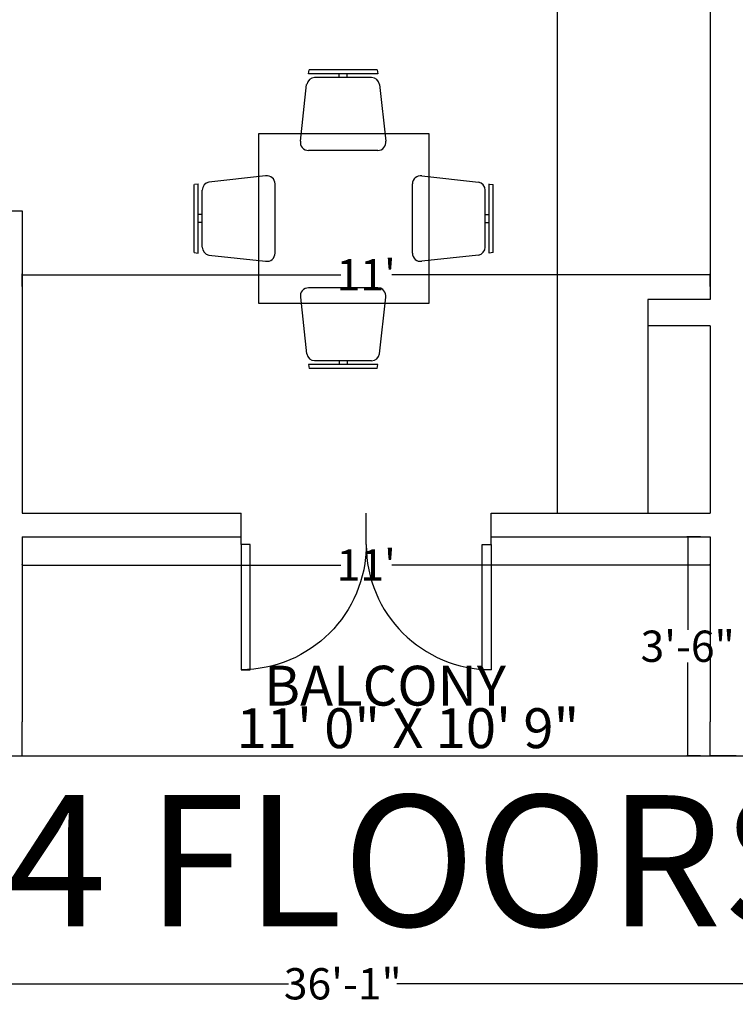
# Model space of a CAD drawing. Units: inches. Extents: x -113 to 5399, y -1393 to 3302.
# Tile 12 of 40: x 1759 to 1896, y 82 to 271. Entities that reach past the tile are written whole.
import ezdxf

# ---------------------------------------------------------------- set-up
doc = ezdxf.new("R2010")
doc.units = ezdxf.units.IN
doc.header["$MEASUREMENT"] = 0
for name, color, linetype, lineweight in [('A-ANNO-DIMS', 254, 'Continuous', 18), ('A-ANNO-TEXT', 7, 'Continuous', 25), ('A-AREA-IDEN', 4, 'Continuous', 18), ('doors', 2, 'Continuous', 25), ('furniture', 131, 'Continuous', 18), ('walls', 1, 'Continuous', 25)]:
    doc.layers.add(name, color=color, linetype=linetype, lineweight=lineweight)
doc.layers.add('B-FURNITURE', color=22, linetype='Continuous')
doc.styles.get("Standard").update_dxf_attribs({"font": 'arial.ttf'})
doc.dimstyles.get("Standard").update_dxf_attribs({"dimtxt": 6, "dimasz": 0.18, "dimexe": 0.18, "dimexo": 0.0625, "dimgap": 0.09, "dimtad": 0, "dimtih": 1, "dimtoh": 1, "dimdec": 1, "dimzin": 0, "dimdsep": 46, "dimlunit": 4, "dimtxsty": 'Standard', "dimblk": 'ARCHTICK', "dimcen": 0.09, "dimadec": 0, "dimazin": 0, "dimtfac": 1, "dimtdec": 1, "dimtofl": 0, "dimtmove": 0, "dimatfit": 3, "dimfxl": 1, "dimtolj": 1, "dimtzin": 0, "dimarcsym": 0})

# ---------------------------------------------------------------- blocks, each defined once
blk = doc.blocks.new('*U2')
for p, q in [((0, 0), (0, -6)), ((24, 0), (24, -6))]:
    blk.add_line(p, q)
blk.add_lwpolyline([(0, 0), (0, 24), (1.75, 24), (1.75, 0)], close=True)
blk.add_arc((0, 0), 24, 0, 90)
blk = doc.blocks.new('A$C6ACA79D1')
at = {"layer": 'B-FURNITURE'}
for p, q in [((-0.5034, 0.0535), (-0.8012, -0.2442)), ((-0.4835, 0.0392), (-0.7869, -0.2642)), ((-0.5034, 0.0535), (-0.4835, 0.0392)), ((-0.4291, 0.0003), (-0.1547, -0.2204)), ((0.7869, -0.259), (0.4835, 0.0444)), ((0.4842, 0.0434), (0.5041, 0.0577)), ((0.7427, -0.249), (0.4935, 0.0002)), ((0.8012, -0.239), (0.5034, 0.0587)), ((-0.4935, -0.005), (-0.7427, -0.2542)), ((-0.601, -0.1125), (-0.6181, -0.0954)), ((0.601, -0.1073), (0.6181, -0.0902)), ((-0.6352, -0.1467), (-0.6523, -0.1296)), ((0.6352, -0.1415), (0.6523, -0.1244)), ((0.8012, -0.239), (0.7869, -0.259)), ((-0.7859, -0.2635), (-0.8002, -0.2436)), ((-0.1485, -0.2964), (-0.4513, -0.5992)), ((0.4513, -0.594), (0.1485, -0.2912)), ((0.748, -0.3133), (0.5273, -0.5877)), ((-0.1485, -1.1937), (-0.4513, -0.8909)), ((0.4513, -0.8961), (0.1485, -1.199)), ((0.748, -1.1768), (0.5273, -0.9024)), ((-0.5034, -1.5436), (-0.8012, -1.2459)), ((-0.7859, -1.2266), (-0.8002, -1.2466)), ((-0.4835, -1.5293), (-0.7869, -1.226)), ((-0.4935, -1.4851), (-0.7427, -1.236)), ((-0.4291, -1.4904), (-0.1547, -1.2698)), ((0.7869, -1.2312), (0.4835, -1.5346)), ((0.7427, -1.2412), (0.4935, -1.4903)), ((0.8012, -1.2511), (0.5034, -1.5488)), ((0.8012, -1.2511), (0.7869, -1.2312)), ((-0.6352, -1.3434), (-0.6523, -1.3605)), ((-0.601, -1.3776), (-0.6181, -1.3948)), ((0.601, -1.3829), (0.6181, -1.4)), ((0.6352, -1.3486), (0.6523, -1.3657)), ((-0.5034, -1.5436), (-0.4835, -1.5293)), ((0.4842, -1.5336), (0.5041, -1.5478))]:
    blk.add_line(p, q, dxfattribs=at)
at = {"layer": 'B-FURNITURE', "ltscale": 300}
for p, q in [((0.1547, -0.2152), (0.4291, 0.0055)), ((-0.5273, -0.593), (-0.748, -0.3186)), ((-0.5273, -0.8972), (-0.748, -1.1716)), ((0.1547, -1.275), (0.4291, -1.4956))]:
    blk.add_line(p, q, dxfattribs=at)
blk.add_lwpolyline([(-0.7425, -0.7425), (0, 0), (0.7425, -0.7425), (0, -1.4849)], close=True, dxfattribs=at)
at = {"layer": 'B-FURNITURE', "ltscale": 400}
for centre, start, end in [((-0.4582, -0.0403), 54.40695, 135), ((0.4589, -0.0361), 45, 125.59305), ((-0.7063, -0.2888), 135, 215.59305), ((0.7073, -0.2843), 324.40695, 45), ((-0.7063, -1.2013), 144.40695, 225), ((0.7073, -1.2059), 315, 35.59305), ((-0.4582, -1.4498), 225, 305.59305), ((0.4589, -1.454), 234.40695, 315)]:
    blk.add_arc(centre, 0.0499, start, end, dxfattribs=at)
at = {"layer": 'B-FURNITURE', "ltscale": 300}
for centre, start, end in [((-0.1838, -0.261), 315, 54.40695), ((0.1838, -0.2558), 125.59305, 225), ((-0.4866, -0.5639), 215.59305, 315), ((0.4866, -0.5586), 225, 324.40695), ((-0.4866, -0.9263), 45, 144.40695), ((0.4866, -0.9315), 35.59305, 135), ((-0.1838, -1.2291), 305.59305, 45), ((0.1838, -1.2343), 135, 234.40695)]:
    blk.add_arc(centre, 0.05, start, end, dxfattribs=at)
blk = doc.blocks.new('_ArchTick')
at = {"color": 0, "linetype": 'ByBlock', "const_width": 0.15}
blk.add_lwpolyline([(-0.5, -0.5), (0.5, 0.5)], dxfattribs=at)
blk = doc.blocks.new('*D59')
at = {"layer": 'A-ANNO-DIMS', "color": 0, "lineweight": -2, "transparency": 16777216}
for p, q in [((1604.26, 136.47), (1604.26, 86.09)), ((2037.26, 136.47), (2037.26, 86.09)), ((1604.26, 86.27), (1810.37, 86.27)), ((2037.26, 86.27), (1831.16, 86.27))]:
    blk.add_line(p, q, dxfattribs=at)
at = {"layer": 'Defpoints', "color": 0, "transparency": 16777216}
for p in [(1604.26, 136.53), (2037.26, 136.53), (2037.26, 86.27)]:
    blk.add_point(p, dxfattribs=at)
at = {"layer": 'A-ANNO-DIMS', "color": 0, "lineweight": -2, "transparency": 16777216, "xscale": 0.18, "yscale": 0.18, "zscale": 0.18, "rotation": 180}
blk.add_blockref('_ArchTick', (1604.26, 86.27), dxfattribs=at)
at = {"layer": 'A-ANNO-DIMS', "color": 0, "lineweight": -2, "transparency": 16777216, "xscale": 0.18, "yscale": 0.18, "zscale": 0.18}
blk.add_blockref('_ArchTick', (2037.26, 86.27), dxfattribs=at)
at = {"layer": 'A-ANNO-DIMS', "color": 0, "transparency": 16777216, "insert": (1820.76, 86.27), "char_height": 6, "attachment_point": 5}
blk.add_mtext('\\A1;36\'-1"', dxfattribs=at)
blk = doc.blocks.new('*D57')
at = {"layer": 'A-ANNO-DIMS', "color": 0, "lineweight": -2, "transparency": 16777216}
for p, q in [((1889.4, 172.03), (1886.75, 172.03)), ((1886.93, 172.03), (1886.93, 154.19)), ((1886.93, 130.03), (1886.93, 147.88)), ((1889.4, 130.03), (1886.75, 130.03))]:
    blk.add_line(p, q, dxfattribs=at)
at = {"layer": 'Defpoints', "color": 0, "transparency": 16777216}
for p in [(1889.46, 172.03), (1886.93, 130.03), (1889.46, 130.03)]:
    blk.add_point(p, dxfattribs=at)
at = {"layer": 'A-ANNO-DIMS', "color": 0, "lineweight": -2, "transparency": 16777216, "xscale": 0.18, "yscale": 0.18, "zscale": 0.18}
for p, rotation in [((1886.93, 172.03), 90), ((1886.93, 130.03), 270)]:
    blk.add_blockref('_ArchTick', p, dxfattribs=dict(at, rotation=rotation))
at = {"layer": 'A-ANNO-DIMS', "color": 0, "transparency": 16777216, "insert": (1886.93, 151.03), "char_height": 6, "attachment_point": 5}
blk.add_mtext('\\A1;3\'-6"', dxfattribs=at)
blk = doc.blocks.new('*D58')
at = {"layer": 'A-ANNO-DIMS', "color": 0, "lineweight": -2, "transparency": 16777216}
for p, q in [((1759.26, 166.68), (1759.26, 166.79)), ((1759.26, 166.61), (1820.36, 166.61)), ((1891.26, 166.61), (1830.16, 166.61)), ((1891.26, 166.68), (1891.26, 166.79))]:
    blk.add_line(p, q, dxfattribs=at)
at = {"layer": 'Defpoints', "color": 0, "transparency": 16777216}
for p in [(1759.26, 166.61), (1891.26, 166.61), (1891.26, 166.61)]:
    blk.add_point(p, dxfattribs=at)
at = {"layer": 'A-ANNO-DIMS', "color": 0, "lineweight": -2, "transparency": 16777216, "xscale": 0.18, "yscale": 0.18, "zscale": 0.18, "rotation": 180}
blk.add_blockref('_ArchTick', (1759.26, 166.61), dxfattribs=at)
at = {"layer": 'A-ANNO-DIMS', "color": 0, "lineweight": -2, "transparency": 16777216, "xscale": 0.18, "yscale": 0.18, "zscale": 0.18}
blk.add_blockref('_ArchTick', (1891.26, 166.61), dxfattribs=at)
at = {"layer": 'A-ANNO-DIMS', "color": 0, "transparency": 16777216, "insert": (1825.26, 166.61), "char_height": 6, "attachment_point": 5}
blk.add_mtext("\\A1;11'", dxfattribs=at)
blk = doc.blocks.new('*D61')
at = {"layer": 'A-ANNO-DIMS', "color": 0, "lineweight": -2, "transparency": 16777216}
for p, q in [((1861.97, 416.53), (1861.97, 299.69)), ((1862.03, 416.53), (1862.15, 416.53)), ((1861.97, 176.53), (1861.97, 293.38)), ((1862.03, 176.53), (1862.15, 176.53))]:
    blk.add_line(p, q, dxfattribs=at)
at = {"layer": 'Defpoints', "color": 0, "transparency": 16777216}
for p in [(1861.97, 416.53), (1861.97, 416.53), (1861.97, 176.53)]:
    blk.add_point(p, dxfattribs=at)
at = {"layer": 'A-ANNO-DIMS', "color": 0, "lineweight": -2, "transparency": 16777216, "xscale": 0.18, "yscale": 0.18, "zscale": 0.18}
for p, rotation in [((1861.97, 416.53), 90), ((1861.97, 176.53), 270)]:
    blk.add_blockref('_ArchTick', p, dxfattribs=dict(at, rotation=rotation))
at = {"layer": 'A-ANNO-DIMS', "color": 0, "transparency": 16777216, "insert": (1861.97, 296.53), "char_height": 6, "attachment_point": 5}
blk.add_mtext("\\A1;20'", dxfattribs=at)
blk = doc.blocks.new('*D62')
at = {"layer": 'A-ANNO-DIMS', "color": 0, "lineweight": -2, "transparency": 16777216}
for p, q in [((1759.26, 220.03), (1759.26, 222.47)), ((1759.26, 222.29), (1820.36, 222.29)), ((1891.26, 222.29), (1830.16, 222.29)), ((1891.26, 220.03), (1891.26, 222.47))]:
    blk.add_line(p, q, dxfattribs=at)
at = {"layer": 'Defpoints', "color": 0, "transparency": 16777216}
for p in [(1759.26, 222.29), (1759.26, 219.97), (1891.26, 219.97)]:
    blk.add_point(p, dxfattribs=at)
at = {"layer": 'A-ANNO-DIMS', "color": 0, "lineweight": -2, "transparency": 16777216, "xscale": 0.18, "yscale": 0.18, "zscale": 0.18, "rotation": 180}
blk.add_blockref('_ArchTick', (1759.26, 222.29), dxfattribs=at)
at = {"layer": 'A-ANNO-DIMS', "color": 0, "lineweight": -2, "transparency": 16777216, "xscale": 0.18, "yscale": 0.18, "zscale": 0.18}
blk.add_blockref('_ArchTick', (1891.26, 222.29), dxfattribs=at)
at = {"layer": 'A-ANNO-DIMS', "color": 0, "transparency": 16777216, "insert": (1825.26, 222.29), "char_height": 6, "attachment_point": 5}
blk.add_mtext("\\A1;11'", dxfattribs=at)
blk = doc.blocks.new('*D209')
at = {"layer": 'A-ANNO-DIMS', "color": 0, "lineweight": -2, "transparency": 16777216}
for p, q in [((1754.32, 798.03), (2074.39, 798.03)), ((2074.21, 798.03), (2074.21, 467.19)), ((2074.21, 130.03), (2074.21, 460.88)), ((1754.32, 130.03), (2074.39, 130.03))]:
    blk.add_line(p, q, dxfattribs=at)
at = {"layer": 'Defpoints', "color": 0, "transparency": 16777216}
for p in [(1754.26, 798.03), (2074.21, 798.03), (1754.26, 130.03)]:
    blk.add_point(p, dxfattribs=at)
at = {"layer": 'A-ANNO-DIMS', "color": 0, "lineweight": -2, "transparency": 16777216, "xscale": 0.18, "yscale": 0.18, "zscale": 0.18}
for p, rotation in [((2074.21, 798.03), 90), ((2074.21, 130.03), 270)]:
    blk.add_blockref('_ArchTick', p, dxfattribs=dict(at, rotation=rotation))
at = {"layer": 'A-ANNO-DIMS', "color": 0, "transparency": 16777216, "insert": (2074.21, 464.03), "char_height": 6, "attachment_point": 5}
blk.add_mtext('\\A1;55\'-8"', dxfattribs=at)

msp = doc.modelspace()

# ---------------------------------------------------------------- linework, layer by layer
at = {"layer": 'walls'}
for p, q in [((1891.26, 292.03), (1891.26, 217.53)), ((1754.26, 234.53), (1759.26, 234.53)), ((1759.26, 234.53), (1759.26, 176.53)), ((1891.26, 217.53), (1879.26, 217.53)), ((1879.26, 217.53), (1879.26, 212.53)), ((1891.26, 212.53), (1879.26, 212.53)), ((1879.26, 212.53), (1879.26, 176.53)), ((1891.26, 212.53), (1891.26, 176.53)), ((1759.26, 176.53), (1801.26, 176.53)), ((1801.26, 172.03), (1801.26, 176.53)), ((1849.26, 176.53), (1891.26, 176.53)), ((1849.26, 172.03), (1849.26, 176.53)), ((1759.26, 172.03), (1759.26, 136.53)), ((1759.26, 172.03), (1801.26, 172.03)), ((1849.26, 172.03), (1891.26, 172.03)), ((1891.26, 172.03), (1891.26, 136.53)), ((1759.26, 130.03), (1759.26, 136.53)), ((1891.26, 130.03), (1891.26, 136.53)), ((1754.26, 130.03), (1759.26, 130.03)), ((1759.26, 130.03), (1891.26, 130.03)), ((1896.26, 130.03), (1891.26, 130.03))]:
    msp.add_line(p, q, dxfattribs=at)

# ---------------------------------------------------------------- block references
at = {"layer": 'doors', "xscale": -1, "rotation": 180}
msp.add_blockref('*U2', (1801.26, 170.53), dxfattribs=at)
at = {"layer": 'doors', "rotation": 180}
msp.add_blockref('*U2', (1849.26, 170.53), dxfattribs=at)
at = {"layer": 'furniture', "xscale": 31.0665876167328, "yscale": 31.0665876167328, "zscale": 31.0665876167328, "rotation": 314.9999999999397}
msp.add_blockref('A$C6ACA79D1', (1837.25, 249.39), dxfattribs=at)

# ---------------------------------------------------------------- texts
at = {"layer": 'A-ANNO-TEXT'}
msp.add_text('1,2,3,4 FLOORS', height=25.17, dxfattribs=at).set_placement((1670.55, 97.29))
at = {"layer": 'A-AREA-IDEN'}
for s, height, p in [('BALCONY', 7.647, (1805.71, 139.64)), ('11\' 0" X 10\' 9"', 7.6473, (1800.38, 131.48))]:
    msp.add_text(s, height=height, dxfattribs=at).set_placement(p)

# ---------------------------------------------------------------- dimensions: what is measured, and where the dimension line sits
at = {"layer": 'A-ANNO-DIMS'}
for base, p1, p2, override, picture, middle in [((2074.21, 798.03), (1754.26, 130.03), (1754.26, 798.03), {"dimdec": 1, "dimlfac": 1, "dimrnd": 0, "dimzin": 1, "dimdsep": 46, "dimlunit": 4, "dimfrac": 2}, '*D209', (2074.21, 464.03)), ((1861.97, 416.53), (1861.97, 176.53), (1861.97, 416.53), {"dimclrd": 0, "dimclre": 0, "dimclrt": 0}, '*D61', (1861.97, 296.53)), ((1886.93, 130.03), (1889.46, 172.03), (1889.46, 130.03), {"dimclrd": 0, "dimclre": 0, "dimclrt": 0}, '*D57', (1886.93, 151.03))]:
    dim = msp.add_linear_dim(base=base, p1=p1, p2=p2, angle=90, dimstyle='Standard', override=override, dxfattribs=at)
    dim.commit()
    dim.dimension.update_dxf_attribs({"geometry": picture, "text_midpoint": middle})
for base, p1, p2, picture, middle in [((1759.26, 222.29), (1891.26, 219.97), (1759.26, 219.97), '*D62', (1825.26, 222.29)), ((1891.26, 166.61), (1759.26, 166.61), (1891.26, 166.61), '*D58', (1825.26, 166.61)), ((2037.26, 86.27), (1604.26, 136.53), (2037.26, 136.53), '*D59', (1820.76, 86.27))]:
    dim = msp.add_linear_dim(base=base, p1=p1, p2=p2, dimstyle='Standard', override={"dimclrd": 0, "dimclre": 0, "dimclrt": 0}, dxfattribs=at)
    dim.commit()
    dim.dimension.update_dxf_attribs({"geometry": picture, "text_midpoint": middle})

doc.saveas('drawing.dxf')
